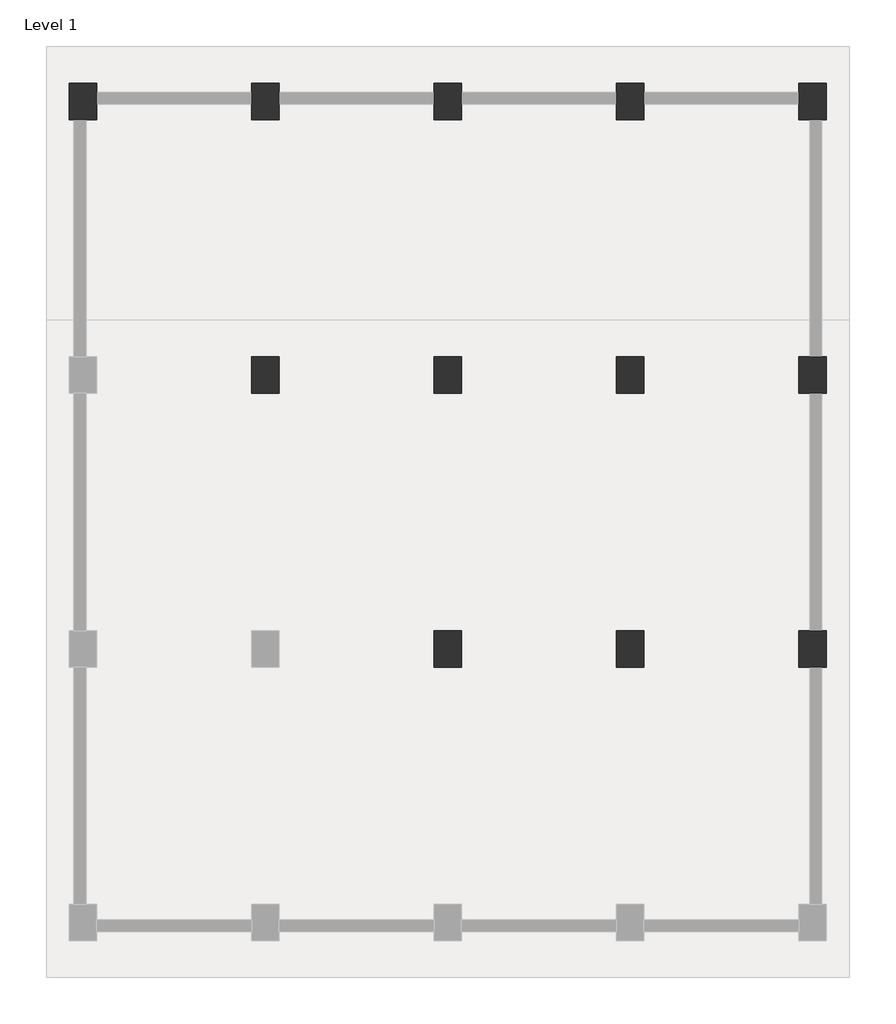
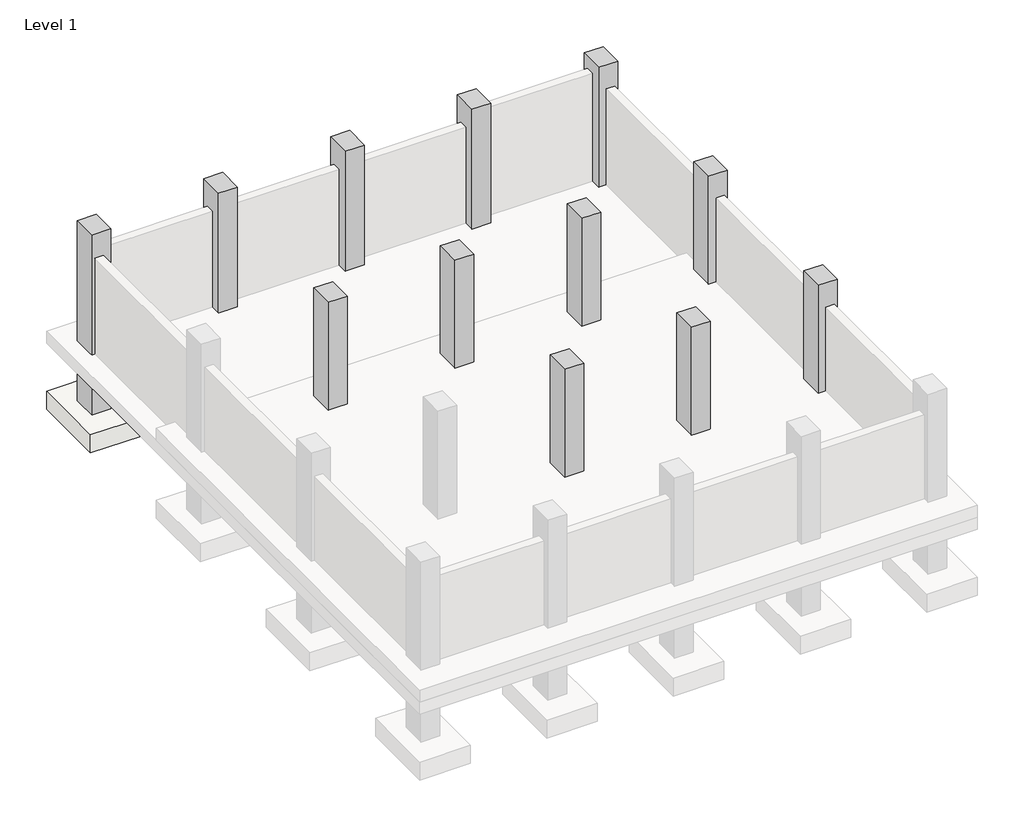
# One storey, part 2 of 2: 19 beams, 12 columns, 12 slabs.
"""IFC4 building model written with IfcOpenShell, lengths in millimetres."""

from ifc_helpers import new_model, si_unit, frame, origin, origin_with_axes, place, context, project, spatial, polyline, outline, extrude, faceted_brep, transform, mapped, element, save
from components import slab_5ba74754

model = new_model("IFC4")

# Units and contexts
model_context = context("Model", 3, world=origin())
ifc_project = project(units=[si_unit("LENGTHUNIT", "METRE", prefix="MILLI")], contexts=[model_context])

# Site, building, storey
site = spatial("IfcSite", under=ifc_project)
building = spatial("IfcBuilding", under=site)
storey = spatial("IfcBuildingStorey", under=building, Name="Level 1", Elevation=0.0)

# Beams
placement = place(None, origin())
element("IfcBeam", 1, ObjectType="Concrete-Rectangular Beam : 12 x 24", at=placement, inside=storey, context=model_context, shape_type="SweptSolid", body=[
    extrude(outline(polyline([(-18724.1183349, 13307.0075069), (-18419.3183349, 13307.0075069), (-18419.3183349, 9344.6075069), (-18724.1183349, 9344.6075069), (-18724.1183349, 13307.0075069)])), frame((0.0, 0.0, -609.6), z_axis=(0.0, 0.0, 1.0), x_axis=(1.0, 0.0, 0.0)), (0.0, 0.0, 1.0), 304.8),
])
element("IfcBeam", 2, ObjectType="Concrete-Rectangular Beam : 12 x 24", at=placement, inside=storey, context=model_context, shape_type="SweptSolid", body=[
    extrude(outline(polyline([(-15676.1183349, 4163.0075069), (-15371.3183349, 4163.0075069), (-15371.3183349, 200.6075069), (-15676.1183349, 200.6075069), (-15676.1183349, 4163.0075069)])), frame((0.0, 0.0, -609.6), z_axis=(0.0, 0.0, 1.0), x_axis=(1.0, 0.0, 0.0)), (0.0, 0.0, 1.0), 304.8),
])
element("IfcBeam", 3, ObjectType="Concrete-Rectangular Beam : 12 x 24", at=placement, inside=storey, context=model_context, shape_type="SweptSolid", body=[
    extrude(outline(polyline([(-15676.1183349, 8735.0075069), (-15371.3183349, 8735.0075069), (-15371.3183349, 4772.6075069), (-15676.1183349, 4772.6075069), (-15676.1183349, 8735.0075069)])), frame((0.0, 0.0, -609.6), z_axis=(0.0, 0.0, 1.0), x_axis=(1.0, 0.0, 0.0)), (0.0, 0.0, 1.0), 304.8),
])
element("IfcBeam", 4, ObjectType="Concrete-Rectangular Beam : 12 x 24", at=placement, inside=storey, context=model_context, shape_type="SweptSolid", body=[
    extrude(outline(polyline([(-15676.1183349, 13307.0075069), (-15371.3183349, 13307.0075069), (-15371.3183349, 9344.6075069), (-15676.1183349, 9344.6075069), (-15676.1183349, 13307.0075069)])), frame((0.0, 0.0, -609.6), z_axis=(0.0, 0.0, 1.0), x_axis=(1.0, 0.0, 0.0)), (0.0, 0.0, 1.0), 304.8),
])
element("IfcBeam", 5, ObjectType="Concrete-Rectangular Beam : 12 x 24", at=placement, inside=storey, context=model_context, shape_type="SweptSolid", body=[
    extrude(outline(polyline([(-12628.1183349, 4163.0075069), (-12323.3183349, 4163.0075069), (-12323.3183349, 200.6075069), (-12628.1183349, 200.6075069), (-12628.1183349, 4163.0075069)])), frame((0.0, 0.0, -609.6), z_axis=(0.0, 0.0, 1.0), x_axis=(1.0, 0.0, 0.0)), (0.0, 0.0, 1.0), 304.8),
])
element("IfcBeam", 6, ObjectType="Concrete-Rectangular Beam : 12 x 24", at=placement, inside=storey, context=model_context, shape_type="SweptSolid", body=[
    extrude(outline(polyline([(-12628.1183349, 8735.0075069), (-12323.3183349, 8735.0075069), (-12323.3183349, 4772.6075069), (-12628.1183349, 4772.6075069), (-12628.1183349, 8735.0075069)])), frame((0.0, 0.0, -609.6), z_axis=(0.0, 0.0, 1.0), x_axis=(1.0, 0.0, 0.0)), (0.0, 0.0, 1.0), 304.8),
])
element("IfcBeam", 7, ObjectType="Concrete-Rectangular Beam : 12 x 24", at=placement, inside=storey, context=model_context, shape_type="SweptSolid", body=[
    extrude(outline(polyline([(-12628.1183349, 13307.0075069), (-12323.3183349, 13307.0075069), (-12323.3183349, 9344.6075069), (-12628.1183349, 9344.6075069), (-12628.1183349, 13307.0075069)])), frame((0.0, 0.0, -609.6), z_axis=(0.0, 0.0, 1.0), x_axis=(1.0, 0.0, 0.0)), (0.0, 0.0, 1.0), 304.8),
])
element("IfcBeam", 8, ObjectType="Concrete-Rectangular Beam : 12 x 24", at=placement, inside=storey, context=model_context, shape_type="SweptSolid", body=[
    extrude(outline(polyline([(-9580.1183349, 4163.0075069), (-9275.3183349, 4163.0075069), (-9275.3183349, 200.6075069), (-9580.1183349, 200.6075069), (-9580.1183349, 4163.0075069)])), frame((0.0, 0.0, -609.6), z_axis=(0.0, 0.0, 1.0), x_axis=(1.0, 0.0, 0.0)), (0.0, 0.0, 1.0), 304.8),
])
element("IfcBeam", 9, ObjectType="Concrete-Rectangular Beam : 12 x 24", at=placement, inside=storey, context=model_context, shape_type="SweptSolid", body=[
    extrude(outline(polyline([(-9580.1183349, 8735.0075069), (-9275.3183349, 8735.0075069), (-9275.3183349, 4772.6075069), (-9580.1183349, 4772.6075069), (-9580.1183349, 8735.0075069)])), frame((0.0, 0.0, -609.6), z_axis=(0.0, 0.0, 1.0), x_axis=(1.0, 0.0, 0.0)), (0.0, 0.0, 1.0), 304.8),
])
element("IfcBeam", 10, ObjectType="Concrete-Rectangular Beam : 12 x 24", at=placement, inside=storey, context=model_context, shape_type="SweptSolid", body=[
    extrude(outline(polyline([(-9580.1183349, 13307.0075069), (-9275.3183349, 13307.0075069), (-9275.3183349, 9344.6075069), (-9580.1183349, 9344.6075069), (-9580.1183349, 13307.0075069)])), frame((0.0, 0.0, -609.6), z_axis=(0.0, 0.0, 1.0), x_axis=(1.0, 0.0, 0.0)), (0.0, 0.0, 1.0), 304.8),
])
element("IfcBeam", 11, ObjectType="Concrete-Rectangular Beam : 12 x 24", at=placement, inside=storey, context=model_context, shape_type="SweptSolid", body=[
    extrude(outline(polyline([(-21391.1183349, 13459.4075069), (-21391.1183349, 13764.2075069), (-18800.3183349, 13764.2075069), (-18800.3183349, 13459.4075069), (-21391.1183349, 13459.4075069)])), frame((0.0, 0.0, -609.6), z_axis=(0.0, 0.0, 1.0), x_axis=(1.0, 0.0, 0.0)), (0.0, 0.0, 1.0), 304.8),
])
element("IfcBeam", 12, ObjectType="Concrete-Rectangular Beam : 12 x 24", at=placement, inside=storey, context=model_context, shape_type="SweptSolid", body=[
    extrude(outline(polyline([(-18343.1183349, 13459.4075069), (-18343.1183349, 13764.2075069), (-15752.3183349, 13764.2075069), (-15752.3183349, 13459.4075069), (-18343.1183349, 13459.4075069)])), frame((0.0, 0.0, -609.6), z_axis=(0.0, 0.0, 1.0), x_axis=(1.0, 0.0, 0.0)), (0.0, 0.0, 1.0), 304.8),
])
element("IfcBeam", 13, ObjectType="Concrete-Rectangular Beam : 12 x 24", at=placement, inside=storey, context=model_context, shape_type="SweptSolid", body=[
    extrude(outline(polyline([(-15295.1183349, 13459.4075069), (-15295.1183349, 13764.2075069), (-12704.3183349, 13764.2075069), (-12704.3183349, 13459.4075069), (-15295.1183349, 13459.4075069)])), frame((0.0, 0.0, -609.6), z_axis=(0.0, 0.0, 1.0), x_axis=(1.0, 0.0, 0.0)), (0.0, 0.0, 1.0), 304.8),
])
element("IfcBeam", 14, ObjectType="Concrete-Rectangular Beam : 12 x 24", at=placement, inside=storey, context=model_context, shape_type="SweptSolid", body=[
    extrude(outline(polyline([(-12247.1183349, 13459.4075069), (-12247.1183349, 13764.2075069), (-9656.3183349, 13764.2075069), (-9656.3183349, 13459.4075069), (-12247.1183349, 13459.4075069)])), frame((0.0, 0.0, -609.6), z_axis=(0.0, 0.0, 1.0), x_axis=(1.0, 0.0, 0.0)), (0.0, 0.0, 1.0), 304.8),
])
element("IfcBeam", 15, ObjectType="Concrete-Rectangular Beam : 12 x 24", at=placement, inside=storey, context=model_context, shape_type="SweptSolid", body=[
    extrude(outline(polyline([(-18343.1183349, 8887.4075069), (-18343.1183349, 9192.2075069), (-15752.3183349, 9192.2075069), (-15752.3183349, 8887.4075069), (-18343.1183349, 8887.4075069)])), frame((0.0, 0.0, -609.6), z_axis=(0.0, 0.0, 1.0), x_axis=(1.0, 0.0, 0.0)), (0.0, 0.0, 1.0), 304.8),
])
element("IfcBeam", 16, ObjectType="Concrete-Rectangular Beam : 12 x 24", at=placement, inside=storey, context=model_context, shape_type="SweptSolid", body=[
    extrude(outline(polyline([(-15295.1183349, 8887.4075069), (-15295.1183349, 9192.2075069), (-12704.3183349, 9192.2075069), (-12704.3183349, 8887.4075069), (-15295.1183349, 8887.4075069)])), frame((0.0, 0.0, -609.6), z_axis=(0.0, 0.0, 1.0), x_axis=(1.0, 0.0, 0.0)), (0.0, 0.0, 1.0), 304.8),
])
element("IfcBeam", 17, ObjectType="Concrete-Rectangular Beam : 12 x 24", at=placement, inside=storey, context=model_context, shape_type="SweptSolid", body=[
    extrude(outline(polyline([(-12247.1183349, 8887.4075069), (-12247.1183349, 9192.2075069), (-9656.3183349, 9192.2075069), (-9656.3183349, 8887.4075069), (-12247.1183349, 8887.4075069)])), frame((0.0, 0.0, -609.6), z_axis=(0.0, 0.0, 1.0), x_axis=(1.0, 0.0, 0.0)), (0.0, 0.0, 1.0), 304.8),
])
element("IfcBeam", 18, ObjectType="Concrete-Rectangular Beam : 12 x 24", at=placement, inside=storey, context=model_context, shape_type="SweptSolid", body=[
    extrude(outline(polyline([(-15295.1183349, 4315.4075069), (-15295.1183349, 4620.2075069), (-12704.3183349, 4620.2075069), (-12704.3183349, 4315.4075069), (-15295.1183349, 4315.4075069)])), frame((0.0, 0.0, -609.6), z_axis=(0.0, 0.0, 1.0), x_axis=(1.0, 0.0, 0.0)), (0.0, 0.0, 1.0), 304.8),
])
element("IfcBeam", 19, ObjectType="Concrete-Rectangular Beam : 12 x 24", at=placement, inside=storey, context=model_context, shape_type="SweptSolid", body=[
    extrude(outline(polyline([(-12247.1183349, 4315.4075069), (-12247.1183349, 4620.2075069), (-9656.3183349, 4620.2075069), (-9656.3183349, 4315.4075069), (-12247.1183349, 4315.4075069)])), frame((0.0, 0.0, -609.6), z_axis=(0.0, 0.0, 1.0), x_axis=(1.0, 0.0, 0.0)), (0.0, 0.0, 1.0), 304.8),
])

# Columns
element("IfcColumn", 20, ObjectType="Concrete-Rectangular-Column : 18 x 24", at=placement, inside=storey, context=model_context, shape_type="Brep", body=[
    faceted_brep([(-21391.1183349, 13916.6075069, -1524.0), (-21391.1183349, 13307.0075069, -1524.0), (-21848.3183349, 13307.0075069, -1524.0), (-21848.3183349, 13916.6075069, -1524.0), (-21391.1183349, 13307.0075069, -304.8), (-21391.1183349, 13916.6075069, -304.8), (-21848.3183349, 13916.6075069, -304.8), (-21848.3183349, 13307.0075069, -304.8)], [[[0, 1, 2, 3]], [[4, 5, 6, 7]], [[1, 0, 5, 4]], [[2, 1, 4, 7]], [[3, 2, 7, 6]], [[0, 3, 6, 5]]]),
    faceted_brep([(-21391.1183349, 13916.6075069, 3048.0), (-21391.1183349, 13307.0075069, 3048.0), (-21391.1183349, 13307.0075069, 0.0), (-21391.1183349, 13561.0075069, 0.0), (-21391.1183349, 13764.2075069, 0.0), (-21391.1183349, 13916.6075069, 0.0), (-21848.3183349, 13307.0075069, 3048.0), (-21848.3183349, 13307.0075069, 0.0), (-21772.1183349, 13307.0075069, 0.0), (-21568.9183349, 13307.0075069, 0.0), (-21848.3183349, 13916.6075069, 3048.0), (-21848.3183349, 13916.6075069, 0.0)], [[[0, 1, 2, 3, 4, 5]], [[1, 6, 7, 8, 9, 2]], [[6, 10, 11, 7]], [[10, 0, 5, 11]], [[1, 0, 10, 6]], [[5, 4, 3, 2, 9, 8, 7, 11]]]),
])
element("IfcColumn", 21, ObjectType="Concrete-Rectangular-Column : 18 x 24", at=placement, inside=storey, context=model_context, shape_type="Brep", body=[
    faceted_brep([(-18343.1183349, 13916.6075069, -1524.0), (-18343.1183349, 13307.0075069, -1524.0), (-18800.3183349, 13307.0075069, -1524.0), (-18800.3183349, 13916.6075069, -1524.0), (-18343.1183349, 13307.0075069, -304.8), (-18343.1183349, 13916.6075069, -304.8), (-18800.3183349, 13916.6075069, -304.8), (-18800.3183349, 13307.0075069, -304.8)], [[[0, 1, 2, 3]], [[4, 5, 6, 7]], [[1, 0, 5, 4]], [[2, 1, 4, 7]], [[3, 2, 7, 6]], [[0, 3, 6, 5]]]),
    faceted_brep([(-18343.1183349, 13916.6075069, 3048.0), (-18343.1183349, 13307.0075069, 3048.0), (-18343.1183349, 13307.0075069, 0.0), (-18343.1183349, 13561.0075069, 0.0), (-18343.1183349, 13764.2075069, 0.0), (-18343.1183349, 13916.6075069, 0.0), (-18800.3183349, 13307.0075069, 3048.0), (-18800.3183349, 13307.0075069, 0.0), (-18800.3183349, 13916.6075069, 3048.0), (-18800.3183349, 13916.6075069, 0.0), (-18800.3183349, 13764.2075069, 0.0), (-18800.3183349, 13561.0075069, 0.0)], [[[0, 1, 2, 3, 4, 5]], [[1, 6, 7, 2]], [[6, 8, 9, 10, 11, 7]], [[8, 0, 5, 9]], [[1, 0, 8, 6]], [[5, 4, 3, 2, 7, 11, 10, 9]]]),
])
element("IfcColumn", 22, ObjectType="Concrete-Rectangular-Column : 18 x 24", at=placement, inside=storey, context=model_context, shape_type="SweptSolid", body=[
    extrude(outline(polyline([(-18343.1183349, 9344.6075069), (-18343.1183349, 8735.0075069), (-18800.3183349, 8735.0075069), (-18800.3183349, 9344.6075069), (-18343.1183349, 9344.6075069)])), frame((0.0, 0.0, -1524.0), z_axis=(0.0, 0.0, 1.0), x_axis=(1.0, 0.0, 0.0)), (0.0, 0.0, 1.0), 1219.2),
    extrude(outline(polyline([(-18343.1183349, 9344.6075069), (-18343.1183349, 8735.0075069), (-18800.3183349, 8735.0075069), (-18800.3183349, 9344.6075069), (-18343.1183349, 9344.6075069)])), origin_with_axes(), (0.0, 0.0, 1.0), 3048.0),
])
element("IfcColumn", 23, ObjectType="Concrete-Rectangular-Column : 18 x 24", at=placement, inside=storey, context=model_context, shape_type="Brep", body=[
    faceted_brep([(-15295.1183349, 13916.6075069, -1524.0), (-15295.1183349, 13307.0075069, -1524.0), (-15752.3183349, 13307.0075069, -1524.0), (-15752.3183349, 13916.6075069, -1524.0), (-15295.1183349, 13307.0075069, -304.8), (-15295.1183349, 13916.6075069, -304.8), (-15752.3183349, 13916.6075069, -304.8), (-15752.3183349, 13307.0075069, -304.8)], [[[0, 1, 2, 3]], [[4, 5, 6, 7]], [[1, 0, 5, 4]], [[2, 1, 4, 7]], [[3, 2, 7, 6]], [[0, 3, 6, 5]]]),
    faceted_brep([(-15295.1183349, 13916.6075069, 3048.0), (-15295.1183349, 13307.0075069, 3048.0), (-15295.1183349, 13307.0075069, 0.0), (-15295.1183349, 13561.0075069, 0.0), (-15295.1183349, 13764.2075069, 0.0), (-15295.1183349, 13916.6075069, 0.0), (-15752.3183349, 13307.0075069, 3048.0), (-15752.3183349, 13307.0075069, 0.0), (-15752.3183349, 13916.6075069, 3048.0), (-15752.3183349, 13916.6075069, 0.0), (-15752.3183349, 13764.2075069, 0.0), (-15752.3183349, 13561.0075069, 0.0)], [[[0, 1, 2, 3, 4, 5]], [[1, 6, 7, 2]], [[6, 8, 9, 10, 11, 7]], [[8, 0, 5, 9]], [[1, 0, 8, 6]], [[5, 4, 3, 2, 7, 11, 10, 9]]]),
])
element("IfcColumn", 24, ObjectType="Concrete-Rectangular-Column : 18 x 24", at=placement, inside=storey, context=model_context, shape_type="SweptSolid", body=[
    extrude(outline(polyline([(-15295.1183349, 9344.6075069), (-15295.1183349, 8735.0075069), (-15752.3183349, 8735.0075069), (-15752.3183349, 9344.6075069), (-15295.1183349, 9344.6075069)])), frame((0.0, 0.0, -1524.0), z_axis=(0.0, 0.0, 1.0), x_axis=(1.0, 0.0, 0.0)), (0.0, 0.0, 1.0), 1219.2),
    extrude(outline(polyline([(-15295.1183349, 9344.6075069), (-15295.1183349, 8735.0075069), (-15752.3183349, 8735.0075069), (-15752.3183349, 9344.6075069), (-15295.1183349, 9344.6075069)])), origin_with_axes(), (0.0, 0.0, 1.0), 3048.0),
])
element("IfcColumn", 25, ObjectType="Concrete-Rectangular-Column : 18 x 24", at=placement, inside=storey, context=model_context, shape_type="SweptSolid", body=[
    extrude(outline(polyline([(-15295.1183349, 4772.6075069), (-15295.1183349, 4163.0075069), (-15752.3183349, 4163.0075069), (-15752.3183349, 4772.6075069), (-15295.1183349, 4772.6075069)])), frame((0.0, 0.0, -1524.0), z_axis=(0.0, 0.0, 1.0), x_axis=(1.0, 0.0, 0.0)), (0.0, 0.0, 1.0), 1219.2),
    extrude(outline(polyline([(-15295.1183349, 4772.6075069), (-15295.1183349, 4163.0075069), (-15752.3183349, 4163.0075069), (-15752.3183349, 4772.6075069), (-15295.1183349, 4772.6075069)])), origin_with_axes(), (0.0, 0.0, 1.0), 3048.0),
])
element("IfcColumn", 26, ObjectType="Concrete-Rectangular-Column : 18 x 24", at=placement, inside=storey, context=model_context, shape_type="Brep", body=[
    faceted_brep([(-12247.1183349, 13916.6075069, -1524.0), (-12247.1183349, 13307.0075069, -1524.0), (-12704.3183349, 13307.0075069, -1524.0), (-12704.3183349, 13916.6075069, -1524.0), (-12247.1183349, 13307.0075069, -304.8), (-12247.1183349, 13916.6075069, -304.8), (-12704.3183349, 13916.6075069, -304.8), (-12704.3183349, 13307.0075069, -304.8)], [[[0, 1, 2, 3]], [[4, 5, 6, 7]], [[1, 0, 5, 4]], [[2, 1, 4, 7]], [[3, 2, 7, 6]], [[0, 3, 6, 5]]]),
    faceted_brep([(-12247.1183349, 13916.6075069, 3048.0), (-12247.1183349, 13307.0075069, 3048.0), (-12247.1183349, 13307.0075069, 0.0), (-12247.1183349, 13561.0075069, 0.0), (-12247.1183349, 13764.2075069, 0.0), (-12247.1183349, 13916.6075069, 0.0), (-12704.3183349, 13307.0075069, 3048.0), (-12704.3183349, 13307.0075069, 0.0), (-12704.3183349, 13916.6075069, 3048.0), (-12704.3183349, 13916.6075069, 0.0), (-12704.3183349, 13764.2075069, 0.0), (-12704.3183349, 13561.0075069, 0.0)], [[[0, 1, 2, 3, 4, 5]], [[1, 6, 7, 2]], [[6, 8, 9, 10, 11, 7]], [[8, 0, 5, 9]], [[1, 0, 8, 6]], [[5, 4, 3, 2, 7, 11, 10, 9]]]),
])
element("IfcColumn", 27, ObjectType="Concrete-Rectangular-Column : 18 x 24", at=placement, inside=storey, context=model_context, shape_type="SweptSolid", body=[
    extrude(outline(polyline([(-12247.1183349, 9344.6075069), (-12247.1183349, 8735.0075069), (-12704.3183349, 8735.0075069), (-12704.3183349, 9344.6075069), (-12247.1183349, 9344.6075069)])), frame((0.0, 0.0, -1524.0), z_axis=(0.0, 0.0, 1.0), x_axis=(1.0, 0.0, 0.0)), (0.0, 0.0, 1.0), 1219.2),
    extrude(outline(polyline([(-12247.1183349, 9344.6075069), (-12247.1183349, 8735.0075069), (-12704.3183349, 8735.0075069), (-12704.3183349, 9344.6075069), (-12247.1183349, 9344.6075069)])), origin_with_axes(), (0.0, 0.0, 1.0), 3048.0),
])
element("IfcColumn", 28, ObjectType="Concrete-Rectangular-Column : 18 x 24", at=placement, inside=storey, context=model_context, shape_type="SweptSolid", body=[
    extrude(outline(polyline([(-12247.1183349, 4772.6075069), (-12247.1183349, 4163.0075069), (-12704.3183349, 4163.0075069), (-12704.3183349, 4772.6075069), (-12247.1183349, 4772.6075069)])), frame((0.0, 0.0, -1524.0), z_axis=(0.0, 0.0, 1.0), x_axis=(1.0, 0.0, 0.0)), (0.0, 0.0, 1.0), 1219.2),
    extrude(outline(polyline([(-12247.1183349, 4772.6075069), (-12247.1183349, 4163.0075069), (-12704.3183349, 4163.0075069), (-12704.3183349, 4772.6075069), (-12247.1183349, 4772.6075069)])), origin_with_axes(), (0.0, 0.0, 1.0), 3048.0),
])
element("IfcColumn", 29, ObjectType="Concrete-Rectangular-Column : 18 x 24", at=placement, inside=storey, context=model_context, shape_type="Brep", body=[
    faceted_brep([(-9199.1183349, 13916.6075069, -1524.0), (-9199.1183349, 13307.0075069, -1524.0), (-9656.3183349, 13307.0075069, -1524.0), (-9656.3183349, 13916.6075069, -1524.0), (-9199.1183349, 13307.0075069, -304.8), (-9199.1183349, 13916.6075069, -304.8), (-9656.3183349, 13916.6075069, -304.8), (-9656.3183349, 13307.0075069, -304.8)], [[[0, 1, 2, 3]], [[4, 5, 6, 7]], [[1, 0, 5, 4]], [[2, 1, 4, 7]], [[3, 2, 7, 6]], [[0, 3, 6, 5]]]),
    faceted_brep([(-9199.1183349, 13916.6075069, 3048.0), (-9199.1183349, 13307.0075069, 3048.0), (-9199.1183349, 13307.0075069, 0.0), (-9199.1183349, 13916.6075069, 0.0), (-9656.3183349, 13307.0075069, 3048.0), (-9656.3183349, 13307.0075069, 0.0), (-9478.5183349, 13307.0075069, 0.0), (-9275.3183349, 13307.0075069, 0.0), (-9656.3183349, 13916.6075069, 3048.0), (-9656.3183349, 13916.6075069, 0.0), (-9656.3183349, 13764.2075069, 0.0), (-9656.3183349, 13561.0075069, 0.0)], [[[0, 1, 2, 3]], [[1, 4, 5, 6, 7, 2]], [[4, 8, 9, 10, 11, 5]], [[8, 0, 3, 9]], [[1, 0, 8, 4]], [[3, 2, 7, 6, 5, 11, 10, 9]]]),
])
element("IfcColumn", 30, ObjectType="Concrete-Rectangular-Column : 18 x 24", at=placement, inside=storey, context=model_context, shape_type="Brep", body=[
    faceted_brep([(-9199.1183349, 9344.6075069, -1524.0), (-9199.1183349, 8735.0075069, -1524.0), (-9656.3183349, 8735.0075069, -1524.0), (-9656.3183349, 9344.6075069, -1524.0), (-9199.1183349, 8735.0075069, -304.8), (-9199.1183349, 9344.6075069, -304.8), (-9656.3183349, 9344.6075069, -304.8), (-9656.3183349, 8735.0075069, -304.8)], [[[0, 1, 2, 3]], [[4, 5, 6, 7]], [[1, 0, 5, 4]], [[2, 1, 4, 7]], [[3, 2, 7, 6]], [[0, 3, 6, 5]]]),
    faceted_brep([(-9199.1183349, 9344.6075069, 3048.0), (-9199.1183349, 8735.0075069, 3048.0), (-9199.1183349, 8735.0075069, 0.0), (-9199.1183349, 9344.6075069, 0.0), (-9656.3183349, 8735.0075069, 3048.0), (-9656.3183349, 8735.0075069, 0.0), (-9478.5183349, 8735.0075069, 0.0), (-9275.3183349, 8735.0075069, 0.0), (-9656.3183349, 9344.6075069, 3048.0), (-9656.3183349, 9344.6075069, 0.0), (-9275.3183349, 9344.6075069, 0.0), (-9478.5183349, 9344.6075069, 0.0)], [[[0, 1, 2, 3]], [[1, 4, 5, 6, 7, 2]], [[4, 8, 9, 5]], [[8, 0, 3, 10, 11, 9]], [[1, 0, 8, 4]], [[3, 2, 7, 6, 5, 9, 11, 10]]]),
])
element("IfcColumn", 31, ObjectType="Concrete-Rectangular-Column : 18 x 24", at=placement, inside=storey, context=model_context, shape_type="Brep", body=[
    faceted_brep([(-9199.1183349, 4772.6075069, -1524.0), (-9199.1183349, 4163.0075069, -1524.0), (-9656.3183349, 4163.0075069, -1524.0), (-9656.3183349, 4772.6075069, -1524.0), (-9199.1183349, 4163.0075069, -304.8), (-9199.1183349, 4772.6075069, -304.8), (-9656.3183349, 4772.6075069, -304.8), (-9656.3183349, 4163.0075069, -304.8)], [[[0, 1, 2, 3]], [[4, 5, 6, 7]], [[1, 0, 5, 4]], [[2, 1, 4, 7]], [[3, 2, 7, 6]], [[0, 3, 6, 5]]]),
    faceted_brep([(-9199.1183349, 4772.6075069, 3048.0), (-9199.1183349, 4163.0075069, 3048.0), (-9199.1183349, 4163.0075069, 0.0), (-9199.1183349, 4772.6075069, 0.0), (-9656.3183349, 4163.0075069, 3048.0), (-9656.3183349, 4163.0075069, 0.0), (-9478.5183349, 4163.0075069, 0.0), (-9275.3183349, 4163.0075069, 0.0), (-9656.3183349, 4772.6075069, 3048.0), (-9656.3183349, 4772.6075069, 0.0), (-9275.3183349, 4772.6075069, 0.0), (-9478.5183349, 4772.6075069, 0.0)], [[[0, 1, 2, 3]], [[1, 4, 5, 6, 7, 2]], [[4, 8, 9, 5]], [[8, 0, 3, 10, 11, 9]], [[1, 0, 8, 4]], [[3, 2, 7, 6, 5, 9, 11, 10]]]),
])

# Slabs
slab_shape = slab_5ba74754(model_context)
element("IfcSlab", 32, ObjectType="Footing-Rectangular : 72\" x 48\" x 18\"", at=placement, inside=storey, context=model_context, shape_type="MappedRepresentation", body=[
    mapped(slab_shape, transform((-21619.7183349, 13611.8075069, -1524.0), x_axis=(1.0, 0.0, 0.0), y_axis=(0.0, 1.0, 0.0), z_axis=(0.0, 0.0, 1.0))),
])
element("IfcSlab", 33, ObjectType="Footing-Rectangular : 72\" x 48\" x 18\"", at=placement, inside=storey, context=model_context, shape_type="MappedRepresentation", body=[
    mapped(slab_shape, transform((-18571.7183349, 13611.8075069, -1524.0), x_axis=(1.0, 0.0, 0.0), y_axis=(0.0, 1.0, 0.0), z_axis=(0.0, 0.0, 1.0))),
])
element("IfcSlab", 34, ObjectType="Footing-Rectangular : 72\" x 48\" x 18\"", at=placement, inside=storey, context=model_context, shape_type="MappedRepresentation", body=[
    mapped(slab_shape, transform((-18571.7183349, 9039.8075069, -1524.0), x_axis=(1.0, 0.0, 0.0), y_axis=(0.0, 1.0, 0.0), z_axis=(0.0, 0.0, 1.0))),
])
element("IfcSlab", 35, ObjectType="Footing-Rectangular : 72\" x 48\" x 18\"", at=placement, inside=storey, context=model_context, shape_type="MappedRepresentation", body=[
    mapped(slab_shape, transform((-15523.7183349, 13611.8075069, -1524.0), x_axis=(1.0, 0.0, 0.0), y_axis=(0.0, 1.0, 0.0), z_axis=(0.0, 0.0, 1.0))),
])
element("IfcSlab", 36, ObjectType="Footing-Rectangular : 72\" x 48\" x 18\"", at=placement, inside=storey, context=model_context, shape_type="MappedRepresentation", body=[
    mapped(slab_shape, transform((-15523.7183349, 9039.8075069, -1524.0), x_axis=(1.0, 0.0, 0.0), y_axis=(0.0, 1.0, 0.0), z_axis=(0.0, 0.0, 1.0))),
])
element("IfcSlab", 37, ObjectType="Footing-Rectangular : 72\" x 48\" x 18\"", at=placement, inside=storey, context=model_context, shape_type="MappedRepresentation", body=[
    mapped(slab_shape, transform((-15523.7183349, 4467.8075069, -1524.0), x_axis=(1.0, 0.0, 0.0), y_axis=(0.0, 1.0, 0.0), z_axis=(0.0, 0.0, 1.0))),
])
element("IfcSlab", 38, ObjectType="Footing-Rectangular : 72\" x 48\" x 18\"", at=placement, inside=storey, context=model_context, shape_type="MappedRepresentation", body=[
    mapped(slab_shape, transform((-12475.7183349, 13611.8075069, -1524.0), x_axis=(1.0, 0.0, 0.0), y_axis=(0.0, 1.0, 0.0), z_axis=(0.0, 0.0, 1.0))),
])
element("IfcSlab", 39, ObjectType="Footing-Rectangular : 72\" x 48\" x 18\"", at=placement, inside=storey, context=model_context, shape_type="MappedRepresentation", body=[
    mapped(slab_shape, transform((-12475.7183349, 9039.8075069, -1524.0), x_axis=(1.0, 0.0, 0.0), y_axis=(0.0, 1.0, 0.0), z_axis=(0.0, 0.0, 1.0))),
])
element("IfcSlab", 40, ObjectType="Footing-Rectangular : 72\" x 48\" x 18\"", at=placement, inside=storey, context=model_context, shape_type="MappedRepresentation", body=[
    mapped(slab_shape, transform((-12475.7183349, 4467.8075069, -1524.0), x_axis=(1.0, 0.0, 0.0), y_axis=(0.0, 1.0, 0.0), z_axis=(0.0, 0.0, 1.0))),
])
element("IfcSlab", 41, ObjectType="Footing-Rectangular : 72\" x 48\" x 18\"", at=placement, inside=storey, context=model_context, shape_type="MappedRepresentation", body=[
    mapped(slab_shape, transform((-9427.7183349, 13611.8075069, -1524.0), x_axis=(1.0, 0.0, 0.0), y_axis=(0.0, 1.0, 0.0), z_axis=(0.0, 0.0, 1.0))),
])
element("IfcSlab", 42, ObjectType="Footing-Rectangular : 72\" x 48\" x 18\"", at=placement, inside=storey, context=model_context, shape_type="MappedRepresentation", body=[
    mapped(slab_shape, transform((-9427.7183349, 9039.8075069, -1524.0), x_axis=(1.0, 0.0, 0.0), y_axis=(0.0, 1.0, 0.0), z_axis=(0.0, 0.0, 1.0))),
])
element("IfcSlab", 43, ObjectType="Footing-Rectangular : 72\" x 48\" x 18\"", at=placement, inside=storey, context=model_context, shape_type="MappedRepresentation", body=[
    mapped(slab_shape, transform((-9427.7183349, 4467.8075069, -1524.0), x_axis=(1.0, 0.0, 0.0), y_axis=(0.0, 1.0, 0.0), z_axis=(0.0, 0.0, 1.0))),
])

save(model, "model.ifc")

# Revit data of these elements
# Type "Concrete-Rectangular Beam : 12 x 24"
#   Assembly Code = "B10"
#   Length [instance default] = 5' - 0"
#   b = 1' - 0"
#   h = 2' - 0"
#   Structural Material [instance default] = Concrete, Cast-in-Place gray
# Type "Concrete-Rectangular-Column : 18 x 24"
#   Assembly Code = "B10"
#   b = 1' - 6"
#   h = 2' - 0"
#   Structural Material [instance default] = Concrete, Cast-in-Place gray
# Type "Footing-Rectangular : 72\" x 48\" x 18\""
#   Assembly Code = "A1010100"
#   Width = 4' - 0"
#   Length = 6' - 0"
#   Foundation Thickness = 1' - 6"
#   Structural Material [instance default] = Concrete, Cast-in-Place gray
# Elements 1, 2, 3, 4, 5, 6, 7, 8, 9, 10, 11, 12, 13, 14, 15, 16, 17, 18, 19 (IfcBeam, "Concrete-Rectangular Beam : 12 x 24")
#   Structural Material = Concrete, Cast-in-Place gray
#   Phase Created = New Construction
#   Materials on its faces: "Concrete, Cast-in-Place gray"
# Elements 20, 21, 22, 23, 24, 25, 26, 27, 28, 29, 30, 31 (IfcColumn, "Concrete-Rectangular-Column : 18 x 24")
#   Structural Material = Concrete, Cast-in-Place gray
#   Phase Created = New Construction
#   Materials on its faces: "Concrete, Cast-in-Place gray"
# Elements 32, 33, 34, 35, 36, 37, 38, 39, 40, 41, 42, 43 (IfcSlab, "Footing-Rectangular : 72\" x 48\" x 18\"")
#   Structural Material = Concrete, Cast-in-Place gray
#   Phase Created = New Construction
#   Materials on its faces: "Concrete, Cast-in-Place gray"
# Materials
#   "Concrete, Cast-in-Place gray": class "Concrete", colour RGB 192 192 192, transparency 0, Description = "Cast-in-place concrete", Cost = 0
